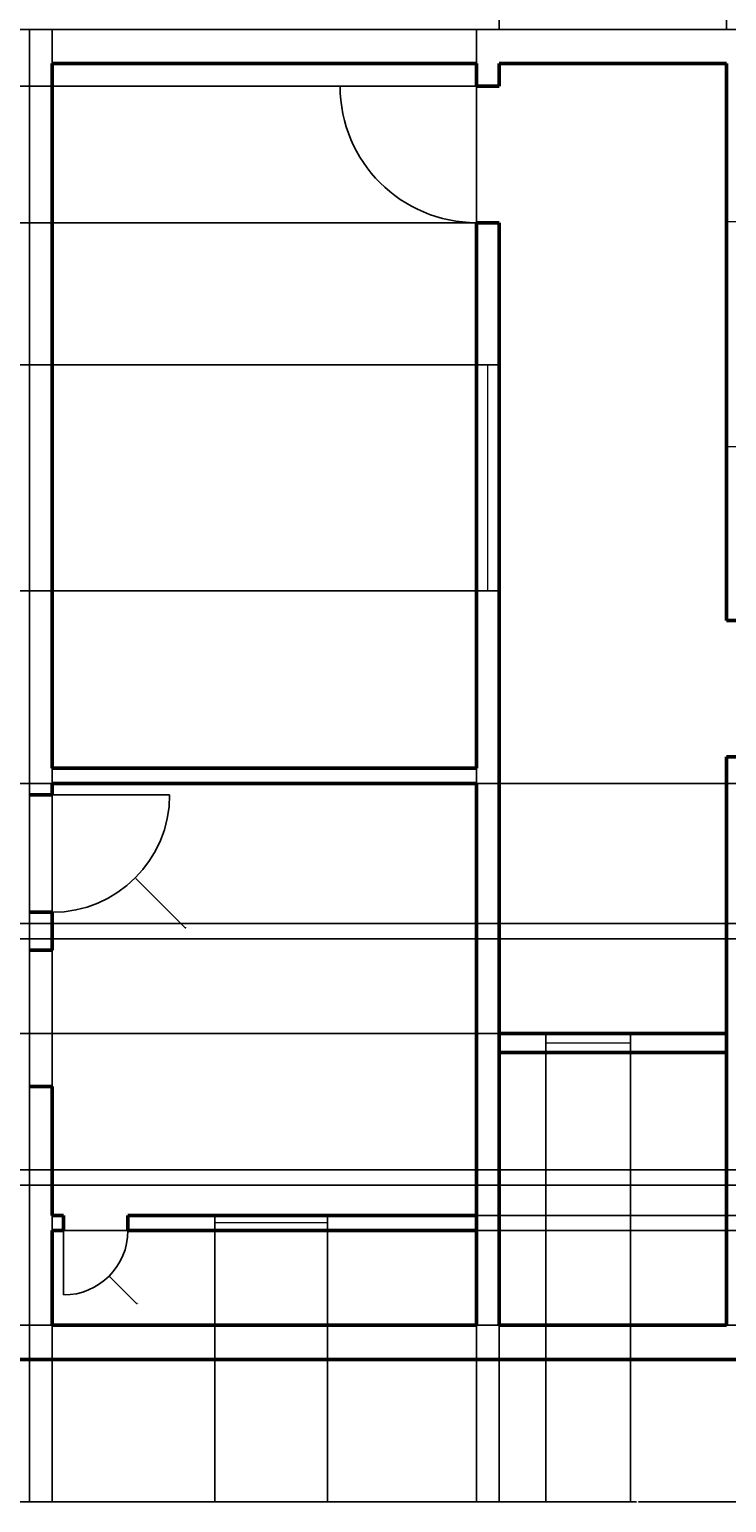
# Model space of a CAD drawing. Units: inches. Extents: x 2479 to 3284, y 2154 to 2936.
# Tile 2 of 8: x 2721 to 2905, y 2154 to 2543. Entities that reach past the tile are written whole.
import ezdxf

# ---------------------------------------------------------------- set-up
doc = ezdxf.new("R2010")
doc.units = ezdxf.units.IN
for name, color, linetype, lineweight in [('A-ANNO-DIMS', 2, 'Continuous', 18), ('A-DOOR', 3, 'Continuous', 25), ('A-GLAZ', 4, 'Continuous', 18), ('A-WALL', 7, 'Continuous', 50)]:
    doc.layers.add(name, color=color, linetype=linetype, lineweight=lineweight)
doc.styles.get("Standard").update_dxf_attribs({"font": 'arial.ttf'})
doc.dimstyles.get("Standard").update_dxf_attribs({"dimtxt": 0.18, "dimasz": 0.18, "dimexe": 0.18, "dimexo": 0.0625, "dimgap": 0.09, "dimtad": 0, "dimtih": 1, "dimtoh": 1, "dimdec": 4, "dimzin": 0, "dimdsep": 46, "dimtxsty": 'Standard', "dimcen": 0.09, "dimadec": 0, "dimazin": 0, "dimtfac": 1, "dimtdec": 4, "dimtofl": 0, "dimtmove": 0, "dimatfit": 3, "dimfxl": 1, "dimtolj": 1, "dimtzin": 0, "dimarcsym": 0})

# ---------------------------------------------------------------- blocks, each defined once
blk = doc.blocks.new('DOOR-SWING-36IN')
blk.add_line((36, 0), (0, 0))
blk.add_arc((36, 0), 36, 90, 180)
blk = doc.blocks.new('*D7')
at = {"layer": 'A-ANNO-DIMS', "color": 0, "lineweight": -2, "transparency": 16777216}
for p, q in [((2517.21, 2191.68), (2517.21, 2153.96)), ((3246.21, 2191.68), (3246.21, 2153.96)), ((2517.39, 2154.14), (2881.42, 2154.14)), ((3246.03, 2154.14), (2882, 2154.14))]:
    blk.add_line(p, q, dxfattribs=at)
at = {"layer": 'A-ANNO-DIMS', "color": 0, "transparency": 16777216}
for points in [[(2517.39, 2154.17), (2517.39, 2154.11), (2517.21, 2154.14)], [(3246.03, 2154.17), (3246.03, 2154.11), (3246.21, 2154.14)]]:
    blk.add_solid(points, dxfattribs=at)
at = {"layer": 'Defpoints', "color": 0, "transparency": 16777216}
for p in [(2517.21, 2191.74), (3246.21, 2191.74), (3246.21, 2154.14)]:
    blk.add_point(p, dxfattribs=at)
at = {"layer": 'A-ANNO-DIMS', "color": 0, "transparency": 16777216, "insert": (2881.71, 2154.14), "char_height": 0.18, "attachment_point": 5}
blk.add_mtext('\\A1;729', dxfattribs=at)
blk = doc.blocks.new('*D11')
at = {"layer": 'A-ANNO-DIMS', "color": 0, "lineweight": -2, "transparency": 16777216}
for p, q in [((2845.21, 2542.8), (2845.21, 2935.52)), ((2845.39, 2935.34), (2874.99, 2935.34)), ((2905.03, 2935.34), (2875.43, 2935.34)), ((2905.21, 2542.8), (2905.21, 2935.52))]:
    blk.add_line(p, q, dxfattribs=at)
at = {"layer": 'A-ANNO-DIMS', "color": 0, "transparency": 16777216}
for points in [[(2845.39, 2935.37), (2845.39, 2935.31), (2845.21, 2935.34)], [(2905.03, 2935.37), (2905.03, 2935.31), (2905.21, 2935.34)]]:
    blk.add_solid(points, dxfattribs=at)
at = {"layer": 'Defpoints', "color": 0, "transparency": 16777216}
for p in [(2905.21, 2935.34), (2845.21, 2542.74), (2905.21, 2542.74)]:
    blk.add_point(p, dxfattribs=at)
at = {"layer": 'A-ANNO-DIMS', "color": 0, "transparency": 16777216, "insert": (2875.21, 2935.34), "char_height": 0.18, "attachment_point": 5}
blk.add_mtext('\\A1;60', dxfattribs=at)
blk = doc.blocks.new('*D12')
at = {"layer": 'A-ANNO-DIMS', "color": 0, "lineweight": -2, "transparency": 16777216}
for p, q in [((2839.21, 2200.68), (2839.21, 2153.96)), ((2845.21, 2200.68), (2845.21, 2153.96)), ((2839.39, 2154.14), (2842.06, 2154.14)), ((2845.03, 2154.14), (2842.36, 2154.14))]:
    blk.add_line(p, q, dxfattribs=at)
at = {"layer": 'A-ANNO-DIMS', "color": 0, "transparency": 16777216}
for points in [[(2839.39, 2154.17), (2839.39, 2154.11), (2839.21, 2154.14)], [(2845.03, 2154.17), (2845.03, 2154.11), (2845.21, 2154.14)]]:
    blk.add_solid(points, dxfattribs=at)
at = {"layer": 'Defpoints', "color": 0, "transparency": 16777216}
for p in [(2839.21, 2200.74), (2845.21, 2200.74), (2845.21, 2154.14)]:
    blk.add_point(p, dxfattribs=at)
at = {"layer": 'A-ANNO-DIMS', "color": 0, "transparency": 16777216, "insert": (2842.21, 2154.14), "char_height": 0.18, "attachment_point": 5}
blk.add_mtext('\\A1;6', dxfattribs=at)
blk = doc.blocks.new('*D15')
at = {"layer": 'A-ANNO-DIMS', "color": 0, "lineweight": -2, "transparency": 16777216}
for p, q in [((2845.21, 2277.68), (2845.21, 2153.96)), ((2857.49, 2277.68), (2857.49, 2153.96)), ((2845.39, 2154.14), (2850.9, 2154.14)), ((2857.31, 2154.14), (2851.81, 2154.14))]:
    blk.add_line(p, q, dxfattribs=at)
at = {"layer": 'A-ANNO-DIMS', "color": 0, "transparency": 16777216}
for points in [[(2845.39, 2154.17), (2845.39, 2154.11), (2845.21, 2154.14)], [(2857.31, 2154.17), (2857.31, 2154.11), (2857.49, 2154.14)]]:
    blk.add_solid(points, dxfattribs=at)
at = {"layer": 'Defpoints', "color": 0, "transparency": 16777216}
for p in [(2845.21, 2277.74), (2857.49, 2277.74), (2857.49, 2154.14)]:
    blk.add_point(p, dxfattribs=at)
at = {"layer": 'A-ANNO-DIMS', "color": 0, "transparency": 16777216, "insert": (2851.35, 2154.14), "char_height": 0.18, "attachment_point": 5}
blk.add_mtext('\\A1;12.284', dxfattribs=at)
blk = doc.blocks.new('*D16')
at = {"layer": 'A-ANNO-DIMS', "color": 0, "lineweight": -2, "transparency": 16777216}
for p, q in [((2857.49, 2277.68), (2857.49, 2153.96)), ((2879.84, 2277.68), (2879.84, 2153.96)), ((2857.67, 2154.14), (2868.27, 2154.14)), ((2879.66, 2154.14), (2869.06, 2154.14))]:
    blk.add_line(p, q, dxfattribs=at)
at = {"layer": 'A-ANNO-DIMS', "color": 0, "transparency": 16777216}
for points in [[(2857.67, 2154.17), (2857.67, 2154.11), (2857.49, 2154.14)], [(2879.66, 2154.17), (2879.66, 2154.11), (2879.84, 2154.14)]]:
    blk.add_solid(points, dxfattribs=at)
at = {"layer": 'Defpoints', "color": 0, "transparency": 16777216}
for p in [(2857.49, 2277.74), (2879.84, 2277.74), (2879.84, 2154.14)]:
    blk.add_point(p, dxfattribs=at)
at = {"layer": 'A-ANNO-DIMS', "color": 0, "transparency": 16777216, "insert": (2868.67, 2154.14), "char_height": 0.18, "attachment_point": 5}
blk.add_mtext('\\A1;22.35', dxfattribs=at)
blk = doc.blocks.new('*D24')
at = {"layer": 'A-ANNO-DIMS', "color": 0, "lineweight": -2, "transparency": 16777216}
for p, q in [((2845.15, 2394.59), (2479.43, 2394.59)), ((2479.61, 2394.41), (2479.61, 2336.35)), ((2479.61, 2277.92), (2479.61, 2335.98)), ((2845.15, 2277.74), (2479.43, 2277.74))]:
    blk.add_line(p, q, dxfattribs=at)
at = {"layer": 'A-ANNO-DIMS', "color": 0, "transparency": 16777216}
for points in [[(2479.58, 2394.41), (2479.64, 2394.41), (2479.61, 2394.59)], [(2479.58, 2277.92), (2479.64, 2277.92), (2479.61, 2277.74)]]:
    blk.add_solid(points, dxfattribs=at)
at = {"layer": 'Defpoints', "color": 0, "transparency": 16777216}
for p in [(2479.61, 2394.59), (2845.21, 2394.59), (2845.21, 2277.74)]:
    blk.add_point(p, dxfattribs=at)
at = {"layer": 'A-ANNO-DIMS', "color": 0, "transparency": 16777216, "insert": (2479.61, 2336.17), "char_height": 0.18, "attachment_point": 5}
blk.add_mtext('\\A1;116.85', dxfattribs=at)
blk = doc.blocks.new('*D25')
at = {"layer": 'A-ANNO-DIMS', "color": 0, "lineweight": -2, "transparency": 16777216}
for p, q in [((2845.15, 2454.21), (2479.43, 2454.21)), ((2479.61, 2454.03), (2479.61, 2424.58)), ((2479.61, 2394.77), (2479.61, 2424.22)), ((2845.15, 2394.59), (2479.43, 2394.59))]:
    blk.add_line(p, q, dxfattribs=at)
at = {"layer": 'A-ANNO-DIMS', "color": 0, "transparency": 16777216}
for points in [[(2479.58, 2454.03), (2479.64, 2454.03), (2479.61, 2454.21)], [(2479.58, 2394.77), (2479.64, 2394.77), (2479.61, 2394.59)]]:
    blk.add_solid(points, dxfattribs=at)
at = {"layer": 'Defpoints', "color": 0, "transparency": 16777216}
for p in [(2479.61, 2454.21), (2845.21, 2454.21), (2845.21, 2394.59)]:
    blk.add_point(p, dxfattribs=at)
at = {"layer": 'A-ANNO-DIMS', "color": 0, "transparency": 16777216, "insert": (2479.61, 2424.4), "char_height": 0.18, "attachment_point": 5}
blk.add_mtext('\\A1;59.61', dxfattribs=at)
blk = doc.blocks.new('*D26')
at = {"layer": 'A-ANNO-DIMS', "color": 0, "lineweight": -2, "transparency": 16777216}
for p, q in [((2845.15, 2491.74), (2479.43, 2491.74)), ((2479.61, 2491.56), (2479.61, 2473.15)), ((2479.61, 2454.39), (2479.61, 2472.79)), ((2845.15, 2454.21), (2479.43, 2454.21))]:
    blk.add_line(p, q, dxfattribs=at)
at = {"layer": 'A-ANNO-DIMS', "color": 0, "transparency": 16777216}
for points in [[(2479.58, 2491.56), (2479.64, 2491.56), (2479.61, 2491.74)], [(2479.58, 2454.39), (2479.64, 2454.39), (2479.61, 2454.21)]]:
    blk.add_solid(points, dxfattribs=at)
at = {"layer": 'Defpoints', "color": 0, "transparency": 16777216}
for p in [(2479.61, 2491.74), (2845.21, 2491.74), (2845.21, 2454.21)]:
    blk.add_point(p, dxfattribs=at)
at = {"layer": 'A-ANNO-DIMS', "color": 0, "transparency": 16777216, "insert": (2479.61, 2472.97), "char_height": 0.18, "attachment_point": 5}
blk.add_mtext('\\A1;37.534', dxfattribs=at)
blk = doc.blocks.new('*D27')
at = {"layer": 'A-ANNO-DIMS', "color": 0, "lineweight": -2, "transparency": 16777216}
for p, q in [((2845.15, 2545.74), (2479.43, 2545.74)), ((2479.61, 2545.56), (2479.61, 2536.92)), ((2479.61, 2527.92), (2479.61, 2536.56)), ((2845.15, 2527.74), (2479.43, 2527.74))]:
    blk.add_line(p, q, dxfattribs=at)
at = {"layer": 'A-ANNO-DIMS', "color": 0, "transparency": 16777216}
for points in [[(2479.58, 2545.56), (2479.64, 2545.56), (2479.61, 2545.74)], [(2479.58, 2527.92), (2479.64, 2527.92), (2479.61, 2527.74)]]:
    blk.add_solid(points, dxfattribs=at)
at = {"layer": 'Defpoints', "color": 0, "transparency": 16777216}
for p in [(2479.61, 2545.74), (2845.21, 2545.74), (2845.21, 2527.74)]:
    blk.add_point(p, dxfattribs=at)
at = {"layer": 'A-ANNO-DIMS', "color": 0, "transparency": 16777216, "insert": (2479.61, 2536.74), "char_height": 0.18, "attachment_point": 5}
blk.add_mtext('\\A1;18', dxfattribs=at)
blk = doc.blocks.new('*D49')
at = {"layer": 'A-ANNO-DIMS', "color": 0, "lineweight": -2, "transparency": 16777216}
for p, q in [((2595.21, 2542.68), (2595.21, 2153.96)), ((2721.21, 2542.68), (2721.21, 2153.96)), ((2595.39, 2154.14), (2657.93, 2154.14)), ((2721.03, 2154.14), (2658.49, 2154.14))]:
    blk.add_line(p, q, dxfattribs=at)
at = {"layer": 'A-ANNO-DIMS', "color": 0, "transparency": 16777216}
for points in [[(2595.39, 2154.17), (2595.39, 2154.11), (2595.21, 2154.14)], [(2721.03, 2154.17), (2721.03, 2154.11), (2721.21, 2154.14)]]:
    blk.add_solid(points, dxfattribs=at)
at = {"layer": 'Defpoints', "color": 0, "transparency": 16777216}
for p in [(2595.21, 2542.74), (2721.21, 2542.74), (2721.21, 2154.14)]:
    blk.add_point(p, dxfattribs=at)
at = {"layer": 'A-ANNO-DIMS', "color": 0, "transparency": 16777216, "insert": (2658.21, 2154.14), "char_height": 0.18, "attachment_point": 5}
blk.add_mtext('\\A1;126', dxfattribs=at)
blk = doc.blocks.new('*D50')
at = {"layer": 'A-ANNO-DIMS', "color": 0, "lineweight": -2, "transparency": 16777216}
for p, q in [((2727.21, 2542.68), (2727.21, 2153.96)), ((2839.21, 2542.68), (2839.21, 2153.96)), ((2727.39, 2154.14), (2782.93, 2154.14)), ((2839.03, 2154.14), (2783.49, 2154.14))]:
    blk.add_line(p, q, dxfattribs=at)
at = {"layer": 'A-ANNO-DIMS', "color": 0, "transparency": 16777216}
for points in [[(2727.39, 2154.17), (2727.39, 2154.11), (2727.21, 2154.14)], [(2839.03, 2154.17), (2839.03, 2154.11), (2839.21, 2154.14)]]:
    blk.add_solid(points, dxfattribs=at)
at = {"layer": 'Defpoints', "color": 0, "transparency": 16777216}
for p in [(2727.21, 2542.74), (2839.21, 2542.74), (2839.21, 2154.14)]:
    blk.add_point(p, dxfattribs=at)
at = {"layer": 'A-ANNO-DIMS', "color": 0, "transparency": 16777216, "insert": (2783.21, 2154.14), "char_height": 0.18, "attachment_point": 5}
blk.add_mtext('\\A1;112', dxfattribs=at)
blk = doc.blocks.new('*D61')
at = {"layer": 'A-ANNO-DIMS', "color": 0, "lineweight": -2, "transparency": 16777216}
for p, q in [((2595.27, 2566.74), (3283.99, 2566.74)), ((3283.81, 2566.56), (3283.81, 2554.92)), ((3283.81, 2542.92), (3283.81, 2554.56)), ((2595.27, 2542.74), (3283.99, 2542.74))]:
    blk.add_line(p, q, dxfattribs=at)
at = {"layer": 'A-ANNO-DIMS', "color": 0, "transparency": 16777216}
for points in [[(3283.78, 2566.56), (3283.84, 2566.56), (3283.81, 2566.74)], [(3283.78, 2542.92), (3283.84, 2542.92), (3283.81, 2542.74)]]:
    blk.add_solid(points, dxfattribs=at)
at = {"layer": 'Defpoints', "color": 0, "transparency": 16777216}
for p in [(2595.21, 2566.74), (3283.81, 2566.74), (2595.21, 2542.74)]:
    blk.add_point(p, dxfattribs=at)
at = {"layer": 'A-ANNO-DIMS', "color": 0, "transparency": 16777216, "insert": (3283.81, 2554.74), "char_height": 0.18, "attachment_point": 5}
blk.add_mtext('\\A1;24', dxfattribs=at)
blk = doc.blocks.new('*D93')
at = {"layer": 'A-ANNO-DIMS', "color": 0, "lineweight": -2, "transparency": 16777216}
for p, q in [((2721.21, 2200.68), (2721.21, 2153.96)), ((2706.69, 2191.68), (2706.69, 2153.96)), ((2706.87, 2154.14), (2713.49, 2154.14)), ((2721.03, 2154.14), (2714.41, 2154.14))]:
    blk.add_line(p, q, dxfattribs=at)
at = {"layer": 'A-ANNO-DIMS', "color": 0, "transparency": 16777216}
for points in [[(2706.87, 2154.17), (2706.87, 2154.11), (2706.69, 2154.14)], [(2721.03, 2154.17), (2721.03, 2154.11), (2721.21, 2154.14)]]:
    blk.add_solid(points, dxfattribs=at)
at = {"layer": 'Defpoints', "color": 0, "transparency": 16777216}
for p in [(2721.21, 2200.74), (2706.69, 2191.74), (2721.21, 2154.14)]:
    blk.add_point(p, dxfattribs=at)
at = {"layer": 'A-ANNO-DIMS', "color": 0, "transparency": 16777216, "insert": (2713.95, 2154.14), "char_height": 0.18, "attachment_point": 5}
blk.add_mtext('\\A1;14.518', dxfattribs=at)
blk = doc.blocks.new('*D94')
at = {"layer": 'A-ANNO-DIMS', "color": 0, "lineweight": -2, "transparency": 16777216}
for p, q in [((2770.18, 2229.68), (2770.18, 2153.96)), ((2799.89, 2229.68), (2799.89, 2153.96)), ((2770.36, 2154.14), (2784.57, 2154.14)), ((2799.71, 2154.14), (2785.5, 2154.14))]:
    blk.add_line(p, q, dxfattribs=at)
at = {"layer": 'A-ANNO-DIMS', "color": 0, "transparency": 16777216}
for points in [[(2770.36, 2154.17), (2770.36, 2154.11), (2770.18, 2154.14)], [(2799.71, 2154.17), (2799.71, 2154.11), (2799.89, 2154.14)]]:
    blk.add_solid(points, dxfattribs=at)
at = {"layer": 'Defpoints', "color": 0, "transparency": 16777216}
for p in [(2770.18, 2229.74), (2799.89, 2229.74), (2799.89, 2154.14)]:
    blk.add_point(p, dxfattribs=at)
at = {"layer": 'A-ANNO-DIMS', "color": 0, "transparency": 16777216, "insert": (2785.04, 2154.14), "char_height": 0.18, "attachment_point": 5}
blk.add_mtext('\\A1;29.717', dxfattribs=at)
blk = doc.blocks.new('*D95')
at = {"layer": 'A-ANNO-DIMS', "color": 0, "lineweight": -2, "transparency": 16777216}
for p, q in [((2799.89, 2229.68), (2799.89, 2153.96)), ((2839.21, 2229.68), (2839.21, 2153.96)), ((2800.07, 2154.14), (2819.09, 2154.14)), ((2839.03, 2154.14), (2820.02, 2154.14))]:
    blk.add_line(p, q, dxfattribs=at)
at = {"layer": 'A-ANNO-DIMS', "color": 0, "transparency": 16777216}
for points in [[(2800.07, 2154.17), (2800.07, 2154.11), (2799.89, 2154.14)], [(2839.03, 2154.17), (2839.03, 2154.11), (2839.21, 2154.14)]]:
    blk.add_solid(points, dxfattribs=at)
at = {"layer": 'Defpoints', "color": 0, "transparency": 16777216}
for p in [(2799.89, 2229.74), (2839.21, 2229.74), (2839.21, 2154.14)]:
    blk.add_point(p, dxfattribs=at)
at = {"layer": 'A-ANNO-DIMS', "color": 0, "transparency": 16777216, "insert": (2819.55, 2154.14), "char_height": 0.18, "attachment_point": 5}
blk.add_mtext('\\A1;39.315', dxfattribs=at)
blk = doc.blocks.new('*D106')
at = {"layer": 'A-ANNO-DIMS', "color": 0, "lineweight": -2, "transparency": 16777216}
for p, q in [((2727.27, 2225.74), (3283.99, 2225.74)), ((3283.81, 2225.56), (3283.81, 2213.42)), ((3283.81, 2200.92), (3283.81, 2213.06)), ((2839.27, 2200.74), (3283.99, 2200.74))]:
    blk.add_line(p, q, dxfattribs=at)
at = {"layer": 'A-ANNO-DIMS', "color": 0, "transparency": 16777216}
for points in [[(3283.78, 2225.56), (3283.84, 2225.56), (3283.81, 2225.74)], [(3283.78, 2200.92), (3283.84, 2200.92), (3283.81, 2200.74)]]:
    blk.add_solid(points, dxfattribs=at)
at = {"layer": 'Defpoints', "color": 0, "transparency": 16777216}
for p in [(2727.21, 2225.74), (3283.81, 2225.74), (2839.21, 2200.74)]:
    blk.add_point(p, dxfattribs=at)
at = {"layer": 'A-ANNO-DIMS', "color": 0, "transparency": 16777216, "insert": (3283.81, 2213.24), "char_height": 0.18, "attachment_point": 5}
blk.add_mtext('\\A1;25', dxfattribs=at)
blk = doc.blocks.new('*D107')
at = {"layer": 'A-ANNO-DIMS', "color": 0, "lineweight": -2, "transparency": 16777216}
for p, q in [((2721.27, 2302.74), (3283.99, 2302.74)), ((3283.81, 2302.56), (3283.81, 2266.42)), ((3283.81, 2229.92), (3283.81, 2266.06)), ((2839.27, 2229.74), (3283.99, 2229.74))]:
    blk.add_line(p, q, dxfattribs=at)
at = {"layer": 'A-ANNO-DIMS', "color": 0, "transparency": 16777216}
for points in [[(3283.78, 2302.56), (3283.84, 2302.56), (3283.81, 2302.74)], [(3283.78, 2229.92), (3283.84, 2229.92), (3283.81, 2229.74)]]:
    blk.add_solid(points, dxfattribs=at)
at = {"layer": 'Defpoints', "color": 0, "transparency": 16777216}
for p in [(2721.21, 2302.74), (2839.21, 2229.74), (3283.81, 2229.74)]:
    blk.add_point(p, dxfattribs=at)
at = {"layer": 'A-ANNO-DIMS', "color": 0, "transparency": 16777216, "insert": (3283.81, 2266.24), "char_height": 0.18, "attachment_point": 5}
blk.add_mtext('\\A1;73', dxfattribs=at)
blk = doc.blocks.new('*D108')
at = {"layer": 'A-ANNO-DIMS', "color": 0, "lineweight": -2, "transparency": 16777216}
for p, q in [((2839.27, 2343.74), (3283.99, 2343.74)), ((3283.81, 2343.56), (3283.81, 2325.42)), ((3283.81, 2306.92), (3283.81, 2325.06)), ((2721.27, 2306.74), (3283.99, 2306.74))]:
    blk.add_line(p, q, dxfattribs=at)
at = {"layer": 'A-ANNO-DIMS', "color": 0, "transparency": 16777216}
for points in [[(3283.78, 2343.56), (3283.84, 2343.56), (3283.81, 2343.74)], [(3283.78, 2306.92), (3283.84, 2306.92), (3283.81, 2306.74)]]:
    blk.add_solid(points, dxfattribs=at)
at = {"layer": 'Defpoints', "color": 0, "transparency": 16777216}
for p in [(2839.21, 2343.74), (3283.81, 2343.74), (2721.21, 2306.74)]:
    blk.add_point(p, dxfattribs=at)
at = {"layer": 'A-ANNO-DIMS', "color": 0, "transparency": 16777216, "insert": (3283.81, 2325.24), "char_height": 0.18, "attachment_point": 5}
blk.add_mtext('\\A1;37', dxfattribs=at)
blk = doc.blocks.new('*D128')
at = {"layer": 'A-ANNO-DIMS', "color": 0, "lineweight": -2, "transparency": 16777216}
for p, q in [((3032.15, 2237.74), (2479.43, 2237.74)), ((2479.61, 2237.56), (2479.61, 2219.42)), ((2479.61, 2200.92), (2479.61, 2219.06)), ((3032.15, 2200.74), (2479.43, 2200.74))]:
    blk.add_line(p, q, dxfattribs=at)
at = {"layer": 'A-ANNO-DIMS', "color": 0, "transparency": 16777216}
for points in [[(2479.58, 2237.56), (2479.64, 2237.56), (2479.61, 2237.74)], [(2479.58, 2200.92), (2479.64, 2200.92), (2479.61, 2200.74)]]:
    blk.add_solid(points, dxfattribs=at)
at = {"layer": 'Defpoints', "color": 0, "transparency": 16777216}
for p in [(2479.61, 2237.74), (3032.21, 2237.74), (3032.21, 2200.74)]:
    blk.add_point(p, dxfattribs=at)
at = {"layer": 'A-ANNO-DIMS', "color": 0, "transparency": 16777216, "insert": (2479.61, 2219.24), "char_height": 0.18, "attachment_point": 5}
blk.add_mtext('\\A1;37', dxfattribs=at)
blk = doc.blocks.new('*D129')
at = {"layer": 'A-ANNO-DIMS', "color": 0, "lineweight": -2, "transparency": 16777216}
for p, q in [((3041.15, 2302.74), (2479.43, 2302.74)), ((2479.61, 2302.56), (2479.61, 2272.42)), ((2479.61, 2241.92), (2479.61, 2272.06)), ((2911.15, 2241.74), (2479.43, 2241.74))]:
    blk.add_line(p, q, dxfattribs=at)
at = {"layer": 'A-ANNO-DIMS', "color": 0, "transparency": 16777216}
for points in [[(2479.58, 2302.56), (2479.64, 2302.56), (2479.61, 2302.74)], [(2479.58, 2241.92), (2479.64, 2241.92), (2479.61, 2241.74)]]:
    blk.add_solid(points, dxfattribs=at)
at = {"layer": 'Defpoints', "color": 0, "transparency": 16777216}
for p in [(2479.61, 2302.74), (3041.21, 2302.74), (2911.21, 2241.74)]:
    blk.add_point(p, dxfattribs=at)
at = {"layer": 'A-ANNO-DIMS', "color": 0, "transparency": 16777216, "insert": (2479.61, 2272.24), "char_height": 0.18, "attachment_point": 5}
blk.add_mtext('\\A1;61', dxfattribs=at)
blk = doc.blocks.new('*D130')
at = {"layer": 'A-ANNO-DIMS', "color": 0, "lineweight": -2, "transparency": 16777216}
for p, q in [((2911.15, 2343.74), (2479.43, 2343.74)), ((2479.61, 2343.56), (2479.61, 2325.42)), ((2479.61, 2306.92), (2479.61, 2325.06)), ((3041.15, 2306.74), (2479.43, 2306.74))]:
    blk.add_line(p, q, dxfattribs=at)
at = {"layer": 'A-ANNO-DIMS', "color": 0, "transparency": 16777216}
for points in [[(2479.58, 2343.56), (2479.64, 2343.56), (2479.61, 2343.74)], [(2479.58, 2306.92), (2479.64, 2306.92), (2479.61, 2306.74)]]:
    blk.add_solid(points, dxfattribs=at)
at = {"layer": 'Defpoints', "color": 0, "transparency": 16777216}
for p in [(2479.61, 2343.74), (2911.21, 2343.74), (3041.21, 2306.74)]:
    blk.add_point(p, dxfattribs=at)
at = {"layer": 'A-ANNO-DIMS', "color": 0, "transparency": 16777216, "insert": (2479.61, 2325.24), "char_height": 0.18, "attachment_point": 5}
blk.add_mtext('\\A1;37', dxfattribs=at)
blk = doc.blocks.new('*D137')
at = {"layer": 'A-ANNO-DIMS', "color": 0, "lineweight": -2, "transparency": 16777216}
for p, q in [((2727.12, 2340.74), (2727.3, 2340.74)), ((2727.21, 2340.65), (2727.21, 2340.83)), ((2762.28, 2305.67), (2749.26, 2318.69)), ((2762.46, 2305.67), (2762.28, 2305.67))]:
    blk.add_line(p, q, dxfattribs=at)
at = {"layer": 'A-ANNO-DIMS', "color": 0, "transparency": 16777216}
blk.add_solid([(2749.28, 2318.71), (2749.23, 2318.67), (2749.13, 2318.82)], dxfattribs=at)
at = {"layer": 'Defpoints', "color": 0, "transparency": 16777216}
for p in [(2727.21, 2340.74), (2749.13, 2318.82)]:
    blk.add_point(p, dxfattribs=at)
at = {"layer": 'A-ANNO-DIMS', "color": 0, "transparency": 16777216, "insert": (2762.75, 2305.67), "char_height": 0.18, "attachment_point": 5}
blk.add_mtext('\\A1;R31', dxfattribs=at)
blk = doc.blocks.new('*D139')
at = {"layer": 'A-ANNO-DIMS', "color": 0, "lineweight": -2, "transparency": 16777216}
for p, q in [((2730.12, 2225.74), (2730.3, 2225.74)), ((2730.21, 2225.65), (2730.21, 2225.83)), ((2749.44, 2206.51), (2742.36, 2213.59)), ((2749.62, 2206.51), (2749.44, 2206.51))]:
    blk.add_line(p, q, dxfattribs=at)
at = {"layer": 'A-ANNO-DIMS', "color": 0, "transparency": 16777216}
blk.add_solid([(2742.38, 2213.61), (2742.34, 2213.57), (2742.23, 2213.72)], dxfattribs=at)
at = {"layer": 'Defpoints', "color": 0, "transparency": 16777216}
for p in [(2730.21, 2225.74), (2742.23, 2213.72)]:
    blk.add_point(p, dxfattribs=at)
at = {"layer": 'A-ANNO-DIMS', "color": 0, "transparency": 16777216, "insert": (2749.93, 2206.51), "char_height": 0.18, "attachment_point": 5}
blk.add_mtext('\\A1;R17', dxfattribs=at)

msp = doc.modelspace()

# ---------------------------------------------------------------- linework, layer by layer
at = {"layer": 'A-DOOR'}
for p, q in [((2727.2088, 2340.7397), (2758.2088, 2340.7397)), ((2730.2088, 2225.7397), (2730.2088, 2208.7397))]:
    msp.add_line(p, q, dxfattribs=at)
for centre, radius in [((2727.2088, 2340.7397), 31), ((2730.2088, 2225.7397), 17)]:
    msp.add_arc(centre, radius, 270, 0, dxfattribs=at)
at = {"layer": 'A-GLAZ'}
for p, q in [((2911.2088, 2491.9355), (2905.2088, 2491.9355)), ((2839.2088, 2454.2054), (2845.2088, 2454.2054)), ((2842.2088, 2394.5937), (2842.2088, 2454.2054)), ((2911.2088, 2432.6017), (2905.2088, 2432.6017)), ((2839.2088, 2394.5937), (2845.2088, 2394.5937)), ((2857.4926, 2277.7397), (2857.4926, 2272.7397)), ((2879.8412, 2275.2397), (2857.4926, 2275.2397)), ((2879.8412, 2277.7397), (2879.8412, 2272.7397)), ((2770.1767, 2229.7397), (2770.1767, 2225.7397)), ((2799.8936, 2227.7397), (2770.1767, 2227.7397)), ((2799.8936, 2229.7397), (2799.8936, 2225.7397))]:
    msp.add_line(p, q, dxfattribs=at)
at = {"layer": 'A-WALL'}
for p, q in [((2727.2088, 2533.7397), (2727.2088, 2347.7397)), ((2839.2088, 2533.7397), (2727.2088, 2533.7397)), ((2839.2088, 2533.7397), (2839.2088, 2527.7397)), ((2845.2088, 2533.7397), (2845.2088, 2527.7397)), ((2905.2088, 2533.7397), (2845.2088, 2533.7397)), ((2905.2088, 2533.7397), (2905.2088, 2386.7397)), ((2839.2088, 2527.7397), (2845.2088, 2527.7397)), ((2839.2088, 2491.7397), (2845.2088, 2491.7397)), ((2839.2088, 2491.7397), (2839.2088, 2347.7397)), ((2845.2088, 2491.7397), (2845.2088, 2200.7397)), ((2911.2088, 2386.7397), (2905.2088, 2386.7397)), ((2911.2088, 2350.7397), (2905.2088, 2350.7397)), ((2905.2088, 2350.7397), (2905.2088, 2200.7397)), ((2839.2088, 2347.7397), (2727.2088, 2347.7397)), ((2727.2088, 2340.7397), (2721.2088, 2340.7397)), ((2839.2088, 2343.7397), (2727.2088, 2343.7397)), ((2727.2088, 2343.7397), (2727.2088, 2340.7397)), ((2839.2088, 2343.7397), (2839.2088, 2200.7397)), ((2721.2088, 2309.7397), (2727.2088, 2309.7397)), ((2727.2088, 2309.7397), (2727.2088, 2299.7397)), ((2721.2088, 2299.7397), (2727.2088, 2299.7397)), ((2845.2088, 2277.7397), (2905.2088, 2277.7397)), ((2845.2088, 2277.7397), (2845.2088, 2272.7397)), ((2845.2088, 2272.7397), (2905.2088, 2272.7397)), ((2721.2088, 2263.7397), (2727.2088, 2263.7397)), ((2727.2088, 2263.7397), (2727.2088, 2229.7397)), ((2730.2088, 2229.7397), (2727.2088, 2229.7397)), ((2730.2088, 2229.7397), (2730.2088, 2225.7397)), ((2839.2088, 2229.7397), (2747.2088, 2229.7397)), ((2747.2088, 2229.7397), (2747.2088, 2225.7397)), ((2730.2088, 2225.7397), (2727.2088, 2225.7397)), ((2727.2088, 2225.7397), (2727.2088, 2200.7397)), ((2839.2088, 2225.7397), (2747.2088, 2225.7397)), ((2727.2088, 2200.7397), (2839.2088, 2200.7397)), ((2845.2088, 2200.7397), (2905.2088, 2200.7397)), ((2517.2088, 2191.7397), (3246.2088, 2191.7397))]:
    msp.add_line(p, q, dxfattribs=at)

# ---------------------------------------------------------------- block references
at = {"layer": 'A-DOOR', "extrusion": (0, 0, -1), "zscale": -1, "rotation": 180}
msp.add_blockref('DOOR-SWING-36IN', (-2803.2088, 2527.7397), dxfattribs=at)

# ---------------------------------------------------------------- dimensions: what is measured, and where the dimension line sits
at = {"layer": 'A-ANNO-DIMS'}
for base, p1, p2, override, picture, middle in [((2905.2088, 2935.3397), (2845.2088, 2542.7397), (2905.2088, 2542.7397), {"dimdec": 0, "dimlfac": 1, "dimrnd": 0, "dimzin": 0, "dimdsep": 46, "dimlunit": 2}, '*D11', (2875.2088, 2935.3397)), ((2721.2088, 2154.1397), (2595.2088, 2542.7397), (2721.2088, 2542.7397), {"dimdec": 0, "dimlfac": 1, "dimrnd": 0, "dimzin": 0, "dimdsep": 46, "dimlunit": 2}, '*D49', (2658.2088, 2154.1397)), ((2839.2088, 2154.1397), (2727.2088, 2542.7397), (2839.2088, 2542.7397), {"dimdec": 0, "dimlfac": 1, "dimrnd": 0, "dimzin": 0, "dimdsep": 46, "dimlunit": 2}, '*D50', (2783.2088, 2154.1397)), ((2857.4926, 2154.1397), (2845.2088, 2277.7397), (2857.4926, 2277.7397), {"dimdec": 3, "dimlfac": 1, "dimrnd": 0, "dimzin": 0, "dimdsep": 46, "dimlunit": 2}, '*D15', (2851.3507, 2154.1397)), ((2879.8412, 2154.1397), (2857.4926, 2277.7397), (2879.8412, 2277.7397), {"dimdec": 2, "dimlfac": 1, "dimrnd": 0, "dimzin": 0, "dimdsep": 46, "dimlunit": 2}, '*D16', (2868.6669, 2154.1397)), ((2799.8936, 2154.1397), (2770.1767, 2229.7397), (2799.8936, 2229.7397), {"dimdec": 3, "dimlfac": 1, "dimrnd": 0, "dimzin": 0, "dimdsep": 46, "dimlunit": 2}, '*D94', (2785.0352, 2154.1397)), ((2839.2088, 2154.1397), (2799.8936, 2229.7397), (2839.2088, 2229.7397), {"dimdec": 3, "dimlfac": 1, "dimrnd": 0, "dimzin": 0, "dimdsep": 46, "dimlunit": 2}, '*D95', (2819.5512, 2154.1397)), ((2721.2088, 2154.1397), (2706.6907, 2191.7397), (2721.2088, 2200.7397), {"dimdec": 3, "dimlfac": 1, "dimrnd": 0, "dimzin": 0, "dimdsep": 46, "dimlunit": 2}, '*D93', (2713.9498, 2154.1397)), ((2845.2088, 2154.1397), (2839.2088, 2200.7397), (2845.2088, 2200.7397), {"dimdec": 0, "dimlfac": 1, "dimrnd": 0, "dimzin": 0, "dimdsep": 46, "dimlunit": 2}, '*D12', (2842.2088, 2154.1397)), ((3246.2088, 2154.1397), (2517.2088, 2191.7397), (3246.2088, 2191.7397), {"dimdec": 0, "dimlfac": 1, "dimrnd": 0, "dimzin": 0, "dimdsep": 46, "dimlunit": 2}, '*D7', (2881.7088, 2154.1397))]:
    dim = msp.add_linear_dim(base=base, p1=p1, p2=p2, dimstyle='Standard', override=override, dxfattribs=at)
    dim.commit()
    dim.dimension.update_dxf_attribs({"geometry": picture, "text_midpoint": middle})
for base, p1, p2, override, picture, middle in [((3283.8088, 2566.7397), (2595.2088, 2542.7397), (2595.2088, 2566.7397), {"dimdec": 0, "dimlfac": 1, "dimrnd": 0, "dimzin": 0, "dimdsep": 46, "dimlunit": 2}, '*D61', (3283.8088, 2554.7397)), ((2479.6088, 2545.7397), (2845.2088, 2527.7397), (2845.2088, 2545.7397), {"dimdec": 0, "dimlfac": 1, "dimrnd": 0, "dimzin": 0, "dimdsep": 46, "dimlunit": 2}, '*D27', (2479.6088, 2536.7397)), ((2479.6088, 2491.7397), (2845.2088, 2454.2054), (2845.2088, 2491.7397), {"dimdec": 3, "dimlfac": 1, "dimrnd": 0, "dimzin": 0, "dimdsep": 46, "dimlunit": 2}, '*D26', (2479.6088, 2472.9726)), ((2479.6088, 2454.2054), (2845.2088, 2394.5937), (2845.2088, 2454.2054), {"dimdec": 2, "dimlfac": 1, "dimrnd": 0, "dimzin": 0, "dimdsep": 46, "dimlunit": 2}, '*D25', (2479.6088, 2424.3996)), ((2479.6088, 2394.5937), (2845.2088, 2277.7397), (2845.2088, 2394.5937), {"dimdec": 2, "dimlfac": 1, "dimrnd": 0, "dimzin": 0, "dimdsep": 46, "dimlunit": 2}, '*D24', (2479.6088, 2336.1667)), ((2479.6088, 2343.7397), (3041.2088, 2306.7397), (2911.2088, 2343.7397), {"dimdec": 0, "dimlfac": 1, "dimrnd": 0, "dimzin": 0, "dimdsep": 46, "dimlunit": 2}, '*D130', (2479.6088, 2325.2397)), ((3283.8088, 2343.7397), (2721.2088, 2306.7397), (2839.2088, 2343.7397), {"dimdec": 0, "dimlfac": 1, "dimrnd": 0, "dimzin": 0, "dimdsep": 46, "dimlunit": 2}, '*D108', (3283.8088, 2325.2397)), ((2479.6088, 2302.7397), (2911.2088, 2241.7397), (3041.2088, 2302.7397), {"dimdec": 0, "dimlfac": 1, "dimrnd": 0, "dimzin": 0, "dimdsep": 46, "dimlunit": 2}, '*D129', (2479.6088, 2272.2397)), ((3283.8088, 2229.7397), (2721.2088, 2302.7397), (2839.2088, 2229.7397), {"dimdec": 0, "dimlfac": 1, "dimrnd": 0, "dimzin": 0, "dimdsep": 46, "dimlunit": 2}, '*D107', (3283.8088, 2266.2397)), ((2479.6088, 2237.7397), (3032.2088, 2200.7397), (3032.2088, 2237.7397), {"dimdec": 0, "dimlfac": 1, "dimrnd": 0, "dimzin": 0, "dimdsep": 46, "dimlunit": 2}, '*D128', (2479.6088, 2219.2397)), ((3283.8088, 2225.7397), (2839.2088, 2200.7397), (2727.2088, 2225.7397), {"dimdec": 0, "dimlfac": 1, "dimrnd": 0, "dimzin": 0, "dimdsep": 46, "dimlunit": 2}, '*D106', (3283.8088, 2213.2397))]:
    dim = msp.add_linear_dim(base=base, p1=p1, p2=p2, angle=90, dimstyle='Standard', override=override, dxfattribs=at)
    dim.commit()
    dim.dimension.update_dxf_attribs({"geometry": picture, "text_midpoint": middle})
for center, mpoint, picture, middle in [((2727.2088, 2340.7397), (2749.1288, 2318.8192), '*D137', (2762.7485, 2305.6668)), ((2730.2088, 2225.7397), (2742.2299, 2213.7191), '*D139', (2749.9275, 2206.5068))]:
    dim = msp.add_radius_dim(center=center, mpoint=mpoint, dimstyle='Standard', override={"dimdec": 0, "dimlfac": 1, "dimrnd": 0, "dimzin": 0, "dimdsep": 46, "dimlunit": 2}, dxfattribs=at)
    dim.commit()
    dim.dimension.update_dxf_attribs({"geometry": picture, "text_midpoint": middle, "dimtype": 164})

doc.saveas('drawing.dxf')
